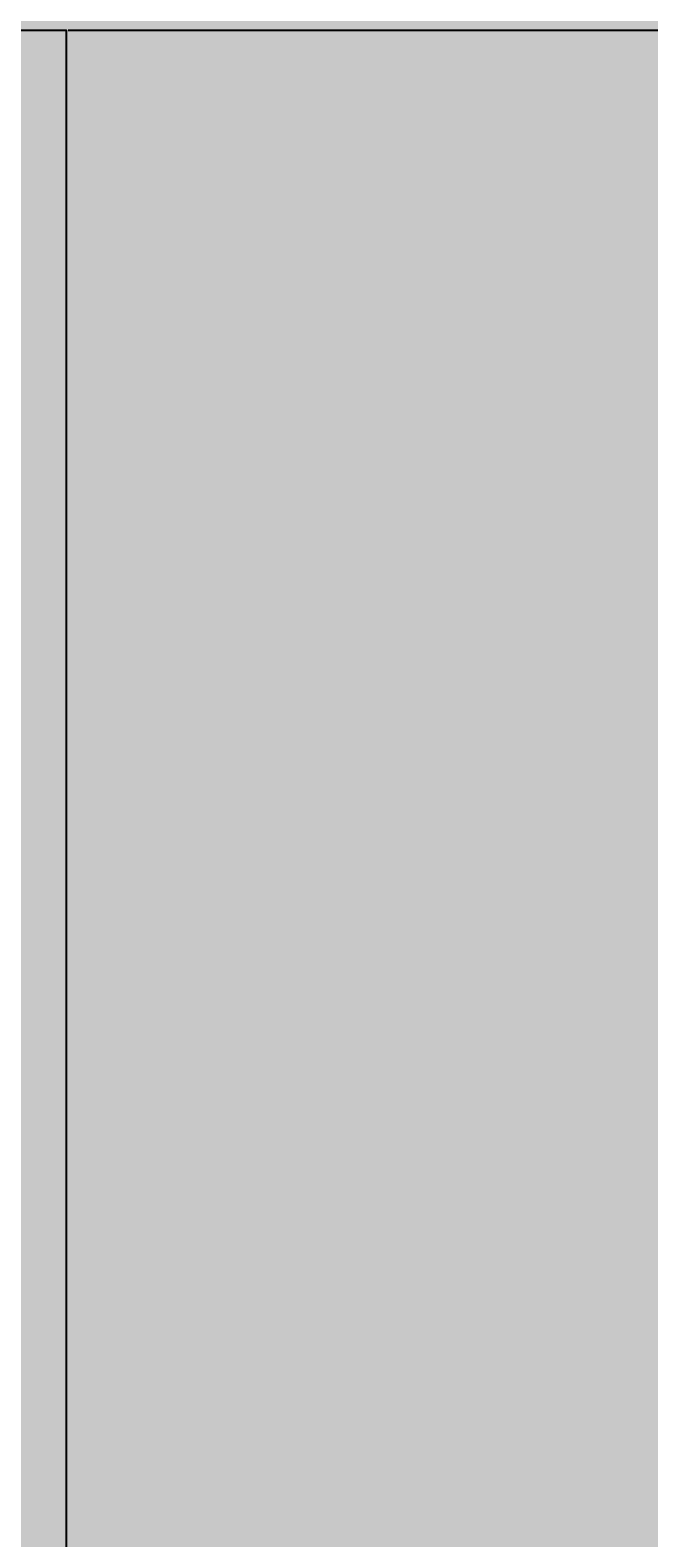
# Model space of a CAD drawing. Units: feet. Extents: x 2695 to 2912, y 795 to 1139.
# Tile 61 of 83: x 2843 to 2860, y 979 to 1021. Entities that reach past the tile are written whole.
import ezdxf

# ---------------------------------------------------------------- set-up
doc = ezdxf.new("R2010")
doc.units = ezdxf.units.FT
for name, color, linetype, lineweight in [('A-ANNO-DIMS', 2, 'Continuous', 18), ('A-ELEV-PATT', 252, 'Continuous', 13), ('A-GLAZ', 4, 'Continuous', 25)]:
    doc.layers.add(name, color=color, linetype=linetype, lineweight=lineweight)
doc.styles.get("Standard").update_dxf_attribs({"font": 'arial.ttf'})
doc.dimstyles.get("Standard").update_dxf_attribs({"dimtxt": 0.18, "dimasz": 0.18, "dimexe": 0.18, "dimexo": 0.0625, "dimgap": 0.09, "dimtad": 0, "dimtih": 1, "dimtoh": 1, "dimdec": 1, "dimzin": 0, "dimdsep": 46, "dimlunit": 3, "dimtxsty": 'Standard', "dimcen": 0.09, "dimadec": 0, "dimazin": 0, "dimtfac": 1, "dimtdec": 1, "dimtofl": 0, "dimtmove": 0, "dimatfit": 3, "dimfxl": 1, "dimtolj": 1, "dimtzin": 0, "dimarcsym": 0})

# ---------------------------------------------------------------- blocks, each defined once
blk = doc.blocks.new('*D17')
at = {"layer": 'A-ANNO-DIMS', "color": 0, "lineweight": -2, "transparency": 16777216}
for p, q in [((2843.637, 1020.824), (2911.424, 1020.824)), ((2911.244, 1020.644), (2911.244, 979.059)), ((2911.244, 937.111), (2911.244, 978.695)), ((2890.699, 936.931), (2911.424, 936.931))]:
    blk.add_line(p, q, dxfattribs=at)
at = {"layer": 'A-ANNO-DIMS', "color": 0, "transparency": 16777216}
for points in [[(2911.214, 1020.644), (2911.274, 1020.644), (2911.244, 1020.824)], [(2911.214, 937.111), (2911.274, 937.111), (2911.244, 936.931)]]:
    blk.add_solid(points, dxfattribs=at)
at = {"layer": 'Defpoints', "color": 0, "transparency": 16777216}
for p in [(2843.575, 1020.824), (2911.244, 1020.824), (2890.636, 936.931)]:
    blk.add_point(p, dxfattribs=at)
at = {"layer": 'A-ANNO-DIMS', "color": 0, "transparency": 16777216, "insert": (2911.244, 978.877), "char_height": 0.18, "attachment_point": 5}
blk.add_mtext('\\A1;83.9', dxfattribs=at)
blk = doc.blocks.new('*D50')
at = {"layer": 'A-ANNO-DIMS', "color": 0, "lineweight": -2, "transparency": 16777216}
for p, q in [((2810.041, 972.03), (2810.041, 1138.886)), ((2888.188, 972.03), (2888.188, 1138.886)), ((2810.221, 1138.706), (2848.721, 1138.706)), ((2888.008, 1138.706), (2849.508, 1138.706))]:
    blk.add_line(p, q, dxfattribs=at)
at = {"layer": 'A-ANNO-DIMS', "color": 0, "transparency": 16777216}
for points in [[(2810.221, 1138.736), (2810.221, 1138.676), (2810.041, 1138.706)], [(2888.008, 1138.736), (2888.008, 1138.676), (2888.188, 1138.706)]]:
    blk.add_solid(points, dxfattribs=at)
at = {"layer": 'Defpoints', "color": 0, "transparency": 16777216}
for p in [(2888.188, 1138.706), (2810.041, 971.967), (2888.188, 971.967)]:
    blk.add_point(p, dxfattribs=at)
at = {"layer": 'A-ANNO-DIMS', "color": 0, "transparency": 16777216, "insert": (2849.114, 1138.706), "char_height": 0.18, "attachment_point": 5}
blk.add_mtext('\\A1;78.15', dxfattribs=at)

msp = doc.modelspace()

# ---------------------------------------------------------------- hatches: boundary and pattern name
at = {"layer": 'A-ELEV-PATT'}
h = msp.add_hatch(color=256, dxfattribs=at)
h.set_gradient(color1=(147, 149, 152), color2=(147, 149, 152), tint=1)
h.paths.add_polyline_path([(2770.6361, 1118.4096), (2710.6361, 1118.4096), (2710.6361, 1062.9306), (2770.6361, 1062.9306)])
h.paths.add_polyline_path([(2890.6361, 1103.3378), (2770.6361, 1103.3378), (2770.6361, 1062.9306), (2890.6361, 1062.9306)])
h.paths.add_polyline_path([(2730.7081, 1048.1052), (2755.1125, 1048.1052), (2755.1125, 936.9306), (2770.6361, 936.9306), (2770.6361, 1050.3105), (2715.8852, 1050.3105), (2715.8852, 936.9306), (2730.7081, 936.9306)])
h.paths.add_polyline_path([(2890.6361, 1050.3105), (2770.6361, 1050.3105), (2770.6361, 971.9673), (2778.0341, 971.9673), (2778.0341, 1020.8235), (2843.575, 1020.8235), (2843.575, 971.9673), (2890.6361, 971.9673)])
h.paths.add_polyline_path([(2888.1882, 970.7156), (2843.575, 970.7156), (2843.575, 964.8267), (2888.1882, 964.8267)])
h.paths.add_polyline_path([(2888.1882, 964.1328), (2843.575, 964.1328), (2843.575, 956.614), (2888.1882, 956.614)])
h.paths.add_polyline_path([(2888.1882, 955.9202), (2843.575, 955.9202), (2843.575, 949.2892), (2888.1882, 949.2892)])
h.paths.add_polyline_path([(2888.1882, 948.5954), (2843.575, 948.5954), (2843.575, 941.3507), (2888.1882, 941.3507)])
h.paths.add_polyline_path([(2888.1882, 940.6569), (2843.575, 940.6569), (2843.575, 936.9306), (2888.1882, 936.9306)])
h.paths.add_polyline_path([(2890.6361, 970.7156), (2888.9368, 970.7156), (2888.9368, 964.8267), (2890.6361, 964.8267)])
h.paths.add_polyline_path([(2890.6361, 964.1328), (2888.9368, 964.1328), (2888.9368, 956.614), (2890.6361, 956.614)])
h.paths.add_polyline_path([(2890.6361, 955.9202), (2888.9368, 955.9202), (2888.9368, 949.2892), (2890.6361, 949.2892)])
h.paths.add_polyline_path([(2890.6361, 940.6569), (2888.9368, 940.6569), (2888.9368, 936.9306), (2890.6361, 936.9306)])
h.paths.add_polyline_path([(2890.6361, 948.5954), (2888.9368, 948.5954), (2888.9368, 941.3507), (2890.6361, 941.3507)])
h.paths.add_polyline_path([(2772.5216, 970.7156), (2770.6361, 970.7156), (2770.6361, 964.8267), (2772.5216, 964.8267)])
h.paths.add_polyline_path([(2772.5216, 964.1328), (2770.6361, 964.1328), (2770.6361, 956.614), (2772.5216, 956.614)])
h.paths.add_polyline_path([(2772.5216, 955.9202), (2770.6361, 955.9202), (2770.6361, 949.2892), (2772.5216, 949.2892)])
h.paths.add_polyline_path([(2772.5216, 948.5954), (2770.6361, 948.5954), (2770.6361, 941.3507), (2772.5216, 941.3507)])
h.paths.add_polyline_path([(2772.5216, 940.6569), (2770.6361, 940.6569), (2770.6361, 936.9306), (2772.5216, 936.9306)])
h.paths.add_polyline_path([(2778.0341, 940.6569), (2773.2702, 940.6569), (2773.2702, 936.9306), (2778.0341, 936.9306)])
h.paths.add_polyline_path([(2778.0341, 970.7156), (2773.2702, 970.7156), (2773.2702, 964.8267), (2778.0341, 964.8267)])
h.paths.add_polyline_path([(2778.0341, 964.1328), (2773.2702, 964.1328), (2773.2702, 956.614), (2778.0341, 956.614)])
h.paths.add_polyline_path([(2778.0341, 955.9202), (2773.2702, 955.9202), (2773.2702, 949.2892), (2778.0341, 949.2892)])
h.paths.add_polyline_path([(2778.0341, 948.5954), (2773.2702, 948.5954), (2773.2702, 941.3507), (2778.0341, 941.3507)])
h.paths.add_polyline_path([(2810.0407, 940.6569), (2780.0341, 940.6569), (2780.0341, 936.9306), (2810.0407, 936.9306)])
h.paths.add_polyline_path([(2890.6361, 924.3105), (2770.6361, 924.3105), (2770.6361, 810.9306), (2773.5029, 810.9306), (2773.5029, 905.5143), (2805.9398, 905.5143), (2838.3767, 905.5143), (2838.3767, 810.9306), (2890.6361, 810.9306)])
h = msp.add_hatch(color=256, dxfattribs=at)
h.set_gradient(color2=(0, 0, 0), tint=1)
h.paths.add_polyline_path([(2772.5216, 971.9673), (2770.6361, 971.9673), (2770.6361, 970.7156), (2772.5216, 970.7156)])
h.paths.add_polyline_path([(2773.2702, 971.9673), (2772.5216, 971.9673), (2772.5216, 970.7156), (2773.2702, 970.7156)])
h.paths.add_polyline_path([(2778.0341, 971.9673), (2773.2702, 971.9673), (2773.2702, 970.7156), (2778.0341, 970.7156)])
h.paths.add_polyline_path([(2780.0341, 971.9673), (2778.0341, 971.9673), (2778.0341, 970.7156), (2780.0341, 970.7156)])
h.paths.add_polyline_path([(2841.575, 971.9673), (2780.0341, 971.9673), (2780.0341, 970.7156), (2841.575, 970.7156)])
h.paths.add_polyline_path([(2843.575, 971.9673), (2841.575, 971.9673), (2841.575, 970.7156), (2843.575, 970.7156)])
h.paths.add_polyline_path([(2888.1882, 971.9673), (2843.575, 971.9673), (2843.575, 970.7156), (2888.1882, 970.7156)])
h.paths.add_polyline_path([(2888.9368, 971.9673), (2888.1882, 971.9673), (2888.1882, 970.7156), (2888.9368, 970.7156)], flags=17)
h.paths.add_polyline_path([(2890.6361, 971.9673), (2888.9368, 971.9673), (2888.9368, 970.7156), (2890.6361, 970.7156)])
h.paths.add_polyline_path([(2888.9368, 971.9673), (2888.1882, 971.9673), (2888.1882, 964.8267), (2888.9368, 964.8267)])
h.paths.add_polyline_path([(2888.9368, 964.8267), (2888.1882, 964.8267), (2888.1882, 964.1328), (2888.9368, 964.1328)])
h.paths.add_polyline_path([(2890.6361, 964.8267), (2888.9368, 964.8267), (2888.9368, 964.1328), (2890.6361, 964.1328)])
h.paths.add_polyline_path([(2888.1882, 964.8267), (2770.6361, 964.8267), (2770.6361, 964.1328), (2888.1882, 964.1328)])
h.paths.add_polyline_path([(2888.9368, 964.1328), (2888.1882, 964.1328), (2888.1882, 936.9306), (2888.9368, 936.9306)])
h.paths.add_polyline_path([(2890.6361, 956.614), (2888.9368, 956.614), (2888.9368, 955.9202), (2890.6361, 955.9202)])
h.paths.add_polyline_path([(2888.1882, 956.614), (2770.6361, 956.614), (2770.6361, 955.9202), (2888.1882, 955.9202)])
h.paths.add_polyline_path([(2890.6361, 949.2892), (2888.9368, 949.2892), (2888.9368, 948.5954), (2890.6361, 948.5954)])
h.paths.add_polyline_path([(2888.1882, 949.2892), (2770.6361, 949.2892), (2770.6361, 948.5954), (2888.1882, 948.5954)])
h.paths.add_polyline_path([(2890.6361, 941.3507), (2888.9368, 941.3507), (2888.9368, 940.6569), (2890.6361, 940.6569)])
h.paths.add_polyline_path([(2888.1882, 941.3507), (2770.6361, 941.3507), (2770.6361, 940.6569), (2888.1882, 940.6569)])
h.paths.add_polyline_path([(2773.2702, 970.7156), (2772.5216, 970.7156), (2772.5216, 964.8267), (2773.2702, 964.8267)])
h.paths.add_polyline_path([(2773.2702, 964.1328), (2772.5216, 964.1328), (2772.5216, 956.614), (2773.2702, 956.614)])
h.paths.add_polyline_path([(2773.2702, 955.9202), (2772.5216, 955.9202), (2772.5216, 936.9306), (2773.2702, 936.9306)])
h.paths.add_polyline_path([(2810.7893, 970.7156), (2810.0407, 970.7156), (2810.0407, 964.8267), (2810.7893, 964.8267)], flags=17)
h.paths.add_polyline_path([(2810.7893, 964.1328), (2810.0407, 964.1328), (2810.0407, 956.614), (2810.7893, 956.614)], flags=17)
h.paths.add_polyline_path([(2810.7893, 955.9202), (2810.0407, 955.9202), (2810.0407, 949.2892), (2810.7893, 949.2892)], flags=17)
h.paths.add_polyline_path([(2810.7893, 971.9673), (2810.0407, 971.9673), (2810.0407, 941.3507), (2810.7893, 941.3507)])
h.paths.add_polyline_path([(2810.7893, 940.6569), (2810.0407, 940.6569), (2810.0407, 936.9306), (2810.7893, 936.9306)])
h.paths.add_polyline_path([(2780.0341, 1018.8235), (2841.575, 1018.8235), (2841.575, 971.9673), (2843.575, 971.9673), (2843.575, 1020.8235), (2778.0341, 1020.8235), (2778.0341, 971.9673), (2780.0341, 971.9673)])
h.paths.add_polyline_path([(2780.0341, 970.7156), (2778.0341, 970.7156), (2778.0341, 964.8267), (2780.0341, 964.8267)])
h.paths.add_polyline_path([(2780.0341, 964.1328), (2778.0341, 964.1328), (2778.0341, 956.614), (2780.0341, 956.614)])
h.paths.add_polyline_path([(2780.0341, 955.9202), (2778.0341, 955.9202), (2778.0341, 949.2892), (2780.0341, 949.2892)])
h.paths.add_polyline_path([(2780.0341, 948.5954), (2778.0341, 948.5954), (2778.0341, 941.3507), (2780.0341, 941.3507)])
h.paths.add_polyline_path([(2780.0341, 940.6569), (2778.0341, 940.6569), (2778.0341, 936.9306), (2780.0341, 936.9306)])
h.paths.add_polyline_path([(2843.575, 940.6569), (2841.575, 940.6569), (2841.575, 936.9306), (2843.575, 936.9306)])
h.paths.add_polyline_path([(2843.575, 948.5954), (2841.575, 948.5954), (2841.575, 941.3507), (2843.575, 941.3507)])
h.paths.add_polyline_path([(2843.575, 970.7156), (2841.575, 970.7156), (2841.575, 964.8267), (2843.575, 964.8267)])
h.paths.add_polyline_path([(2843.575, 964.1328), (2841.575, 964.1328), (2841.575, 956.614), (2843.575, 956.614)])
h.paths.add_polyline_path([(2843.575, 955.9202), (2841.575, 955.9202), (2841.575, 949.2892), (2843.575, 949.2892)])
h.paths.add_polyline_path([(2805.0538, 874.1057), (2803.9681, 874.1057), (2803.9681, 846.2857), (2805.0538, 846.2857)])
h.paths.add_polyline_path([(2758.1515, 902.577), (2724.1893, 902.577), (2724.1893, 874.8571), (2758.1515, 874.8571)])
h.paths.add_polyline_path([(2726.1893, 900.577), (2756.1515, 900.577), (2756.1515, 876.8571), (2726.1893, 876.8571)], flags=16)
h.paths.add_polyline_path([(2740.7302, 900.577), (2741.6105, 900.577), (2741.6105, 876.8571), (2740.7302, 876.8571)], flags=0)

# ---------------------------------------------------------------- linework, layer by layer
at = {"layer": 'A-GLAZ'}
msp.add_lwpolyline([(2778.0341, 936.9306), (2778.0341, 1020.8235), (2843.575, 1020.8235), (2843.575, 936.9306)], dxfattribs=at)

# ---------------------------------------------------------------- dimensions: what is measured, and where the dimension line sits
at = {"layer": 'A-ANNO-DIMS'}
dim = msp.add_linear_dim(base=(2888.1882, 1138.7056), p1=(2810.0407, 971.9673), p2=(2888.1882, 971.9673), dimstyle='Standard', override={"dimdec": 2, "dimlfac": 1, "dimrnd": 0, "dimzin": 0, "dimdsep": 46, "dimlunit": 2}, dxfattribs=at)
dim.commit()
dim.dimension.update_dxf_attribs({"geometry": '*D50', "text_midpoint": (2849.1144, 1138.7056)})
dim = msp.add_linear_dim(base=(2911.2444, 1020.8235), p1=(2890.6361, 936.9306), p2=(2843.575, 1020.8235), angle=90, dimstyle='Standard', override={"dimdec": 1, "dimlfac": 1, "dimrnd": 0, "dimzin": 0, "dimdsep": 46, "dimlunit": 2}, dxfattribs=at)
dim.commit()
dim.dimension.update_dxf_attribs({"geometry": '*D17', "text_midpoint": (2911.2444, 978.877)})

doc.saveas('drawing.dxf')
